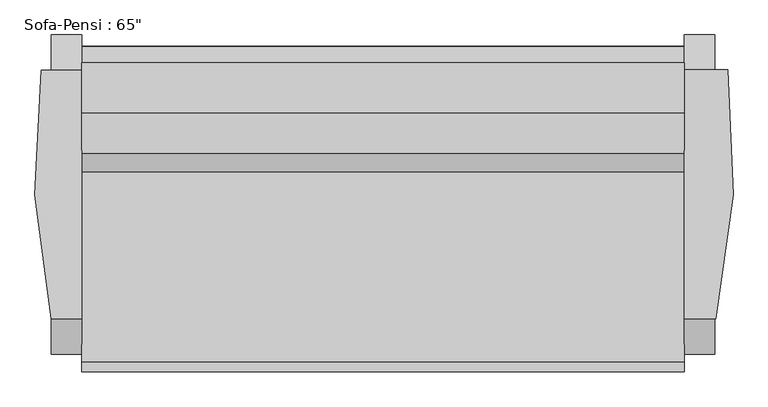
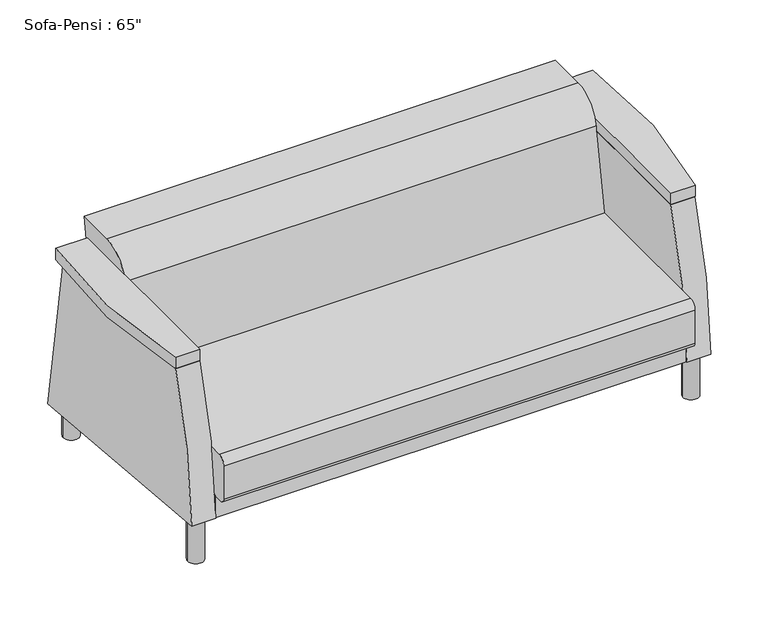
"""IFC4 building model written with IfcOpenShell, lengths in millimetres: furniture geometry."""

from ifc_helpers import new_model, si_unit, point, frame, frame_2d, origin, origin_with_axes, place, context, project, spatial, polyline, circle_curve, trimmed, segment, composite_curve, outline, extrude, source, transform, mapped, element, save


def furniture_ad7727fe(model_context):
    return source(origin(), model_context, "Body", "SweptSolid", [
        extrude(outline(composite_curve([segment(trimmed(circle_curve(frame_2d((-508.79375, -53.0901639)), 25.4), [point((-534.19375, -53.0901639))], [point((-483.39375, -53.0901639))], False, "CARTESIAN"), True, "CONTINUOUS"), segment(trimmed(circle_curve(frame_2d((-508.79375, -53.0901639)), 25.4), [point((-483.39375, -53.0901639))], [point((-534.19375, -53.0901639))], False, "CARTESIAN"), True, "CONTINUOUS")], self_intersect=False)), origin_with_axes(), (0.0, 0.0, 1.0), 148.43125),
        extrude(outline(composite_curve([segment(trimmed(circle_curve(frame_2d((-508.79375, 632.7098361)), 25.4), [point((-534.19375, 632.7098361))], [point((-483.39375, 632.7098361))], False, "CARTESIAN"), True, "CONTINUOUS"), segment(trimmed(circle_curve(frame_2d((-508.79375, 632.7098361)), 25.4), [point((-483.39375, 632.7098361))], [point((-534.19375, 632.7098361))], False, "CARTESIAN"), True, "CONTINUOUS")], self_intersect=False)), origin_with_axes(), (0.0, 0.0, 1.0), 148.43125),
        extrude(outline(composite_curve([segment(trimmed(circle_curve(frame_2d((1066.00625, 632.7098361)), 25.4), [point((1040.60625, 632.7098361))], [point((1091.40625, 632.7098361))], False, "CARTESIAN"), True, "CONTINUOUS"), segment(trimmed(circle_curve(frame_2d((1066.00625, 632.7098361)), 25.4), [point((1091.40625, 632.7098361))], [point((1040.60625, 632.7098361))], False, "CARTESIAN"), True, "CONTINUOUS")], self_intersect=False)), origin_with_axes(), (0.0, 0.0, 1.0), 148.43125),
        extrude(outline(composite_curve([segment(trimmed(circle_curve(frame_2d((1066.00625, -53.0901639)), 25.4), [point((1040.60625, -53.0901639))], [point((1091.40625, -53.0901639))], False, "CARTESIAN"), True, "CONTINUOUS"), segment(trimmed(circle_curve(frame_2d((1066.00625, -53.0901639)), 25.4), [point((1091.40625, -53.0901639))], [point((1040.60625, -53.0901639))], False, "CARTESIAN"), True, "CONTINUOUS")], self_intersect=False)), origin_with_axes(), (0.0, 0.0, 1.0), 148.43125),
        extrude(outline(polyline([(1027.90625, 668.3047863), (1027.90625, -93.6952137), (-470.69375, -93.6952137), (-470.69375, 668.3047863), (1027.90625, 668.3047863)])), frame((0.0, 0.0, 148.0509954), z_axis=(0.0, 0.0, 1.0), x_axis=(1.0, 0.0, 0.0)), (0.0, 0.0, 1.0), 76.2),
        extrude(outline(composite_curve([segment(polyline([(-9.3943348, 626.0203985), (608.6917937, 626.0203985), (696.2098361, 79.844579), (-97.7900405, 149.3105671)]), True, "CONTINUOUS"), segment(trimmed(circle_curve(frame_2d((1499.9783711, 99.5888442)), 1598.5418814), [point((-97.7900405, 149.3105671))], [point((-9.3943348, 626.0203985))], False, "CARTESIAN"), True, "CONTINUOUS")], self_intersect=False)), frame((-546.89375, 0.0, 0.0), z_axis=(1.0, 0.0, 0.0), x_axis=(0.0, 1.0, 0.0)), (0.0, 0.0, 1.0), 76.2),
        extrude(outline(composite_curve([segment(polyline([(696.2098361, 79.844579), (-97.7900405, 149.3105671)]), True, "CONTINUOUS"), segment(trimmed(circle_curve(frame_2d((1499.9783711, 99.5888442)), 1598.5418814), [point((-97.7900405, 149.3105671))], [point((-9.3943348, 626.0203985))], False, "CARTESIAN"), True, "CONTINUOUS"), segment(polyline([(-9.3943348, 626.0203985), (608.6917937, 626.0203985), (696.2098361, 79.844579)]), True, "CONTINUOUS")], self_intersect=False)), frame((1027.90625, 0.0, 0.0), z_axis=(1.0, 0.0, 0.0), x_axis=(0.0, 1.0, 0.0)), (0.0, 0.0, 1.0), 76.2),
        extrude(outline(composite_curve([segment(trimmed(circle_curve(frame_2d((-116.5901639, 351.2509954)), 25.4), [point((-141.9901639, 351.2509954))], [point((-116.5901639, 376.6509954))], False, "CARTESIAN"), True, "CONTINUOUS"), segment(polyline([(-116.5901639, 376.6509954), (355.3895541, 376.6509954), (402.1988177, 642.1195211)]), True, "CONTINUOUS"), segment(trimmed(circle_curve(frame_2d((502.2552854, 624.4768662)), 101.6), [point((402.1988177, 642.1195211))], [point((502.2552854, 726.0768662))], False, "CARTESIAN"), True, "CONTINUOUS"), segment(polyline([(502.2552854, 726.0768662), (626.3344485, 726.0768662), (609.5377828, 620.1719187), (667.6541767, 224.2509954), (-126.1151639, 224.2509954)]), True, "CONTINUOUS"), segment(trimmed(circle_curve(frame_2d((-126.1151639, 240.1259954)), 15.875), [point((-126.1151639, 224.2509954))], [point((-141.9901639, 240.1259954))], False, "CARTESIAN"), True, "CONTINUOUS"), segment(polyline([(-141.9901639, 240.1259954), (-141.9901639, 351.2509954)]), True, "CONTINUOUS")], self_intersect=False)), frame((-470.69375, 0.0, 0.0), z_axis=(1.0, 0.0, 0.0), x_axis=(0.0, 1.0, 0.0)), (0.0, 0.0, 1.0), 1498.6),
        extrude(outline(composite_curve([segment(polyline([(-470.69375, -9.3943348), (-546.89375, -9.3943348)]), True, "CONTINUOUS"), segment(trimmed(circle_curve(frame_2d((1138.2527561, 369.4210463)), 1727.2), [point((-546.89375, -9.3943348))], [point((-572.29375, 608.6917935))], False, "CARTESIAN"), True, "CONTINUOUS"), segment(polyline([(-572.29375, 608.6917935), (-470.69375, 608.6917935), (-470.69375, -9.3943348)]), True, "CONTINUOUS")], self_intersect=False)), frame((0.0, 0.0, 626.0203985), z_axis=(0.0, 0.0, 1.0), x_axis=(1.0, 0.0, 0.0)), (0.0, 0.0, 1.0), 38.1),
        extrude(outline(composite_curve([segment(polyline([(1027.90625, -9.3943348), (1027.90625, 608.9395268), (1136.5864453, 608.9395268)]), True, "CONTINUOUS"), segment(trimmed(circle_curve(frame_2d((-580.0771494, 383.3125476)), 1731.4275703), [point((1136.5864453, 608.9395268))], [point((1106.2273117, -9.3943348))], False, "CARTESIAN"), True, "CONTINUOUS"), segment(polyline([(1106.2273117, -9.3943348), (1027.90625, -9.3943348)]), True, "CONTINUOUS")], self_intersect=False)), frame((0.0, 0.0, 626.0203985), z_axis=(0.0, 0.0, 1.0), x_axis=(1.0, 0.0, 0.0)), (0.0, 0.0, 1.0), 38.1),
    ])


if __name__ == "__main__":
    model = new_model("IFC4")
    model_context = context("Model", 3, world=origin())
    ifc_project = project(units=[si_unit("LENGTHUNIT", "METRE", prefix="MILLI")], contexts=[model_context])
    site = spatial("IfcSite", under=ifc_project)
    building = spatial("IfcBuilding", under=site)
    placement = place(None, origin())
    furniture_shape = furniture_ad7727fe(model_context)
    element("IfcFurniture", 1, ObjectType="Sofa-Pensi : 65\"", at=placement, inside=building, context=model_context, shape_type="MappedRepresentation", body=[
        mapped(furniture_shape, transform((0.0, 0.0, 0.0), x_axis=(1.0, 0.0, 0.0), y_axis=(0.0, 1.0, 0.0), z_axis=(0.0, 0.0, 1.0))),
    ])
    save(model, "model.ifc")

# Revit data of these elements
# Type "Sofa-Pensi : 65\""
#   Assembly Code = "E2020200"
#   Length = 5' - 5"
#   Frame Material = Cherry
#   Seat Material = Linen, Beige
#   Feet Material = Steel, Chrome Plated
#   Default Elevation = 0
# Element 1 (IfcFurniture, "Sofa-Pensi : 65\"")
#   Materials on its faces: "Cherry", "Linen, Beige", "Steel, Chrome Plated"
# Materials
#   "Cherry": class "Wood", colour RGB 226 177 128, transparency 0, Description = "Prunus Serotina", Cost = 0
#   "Linen, Beige": class "Textile", colour RGB 249 239 230, transparency 0, Description = "Linen, beige", Cost = 0
#   "Steel, Chrome Plated": class "Metal", colour RGB 17 17 17, transparency 0, Description = "Chromiuim plated steel", Cost = 0
